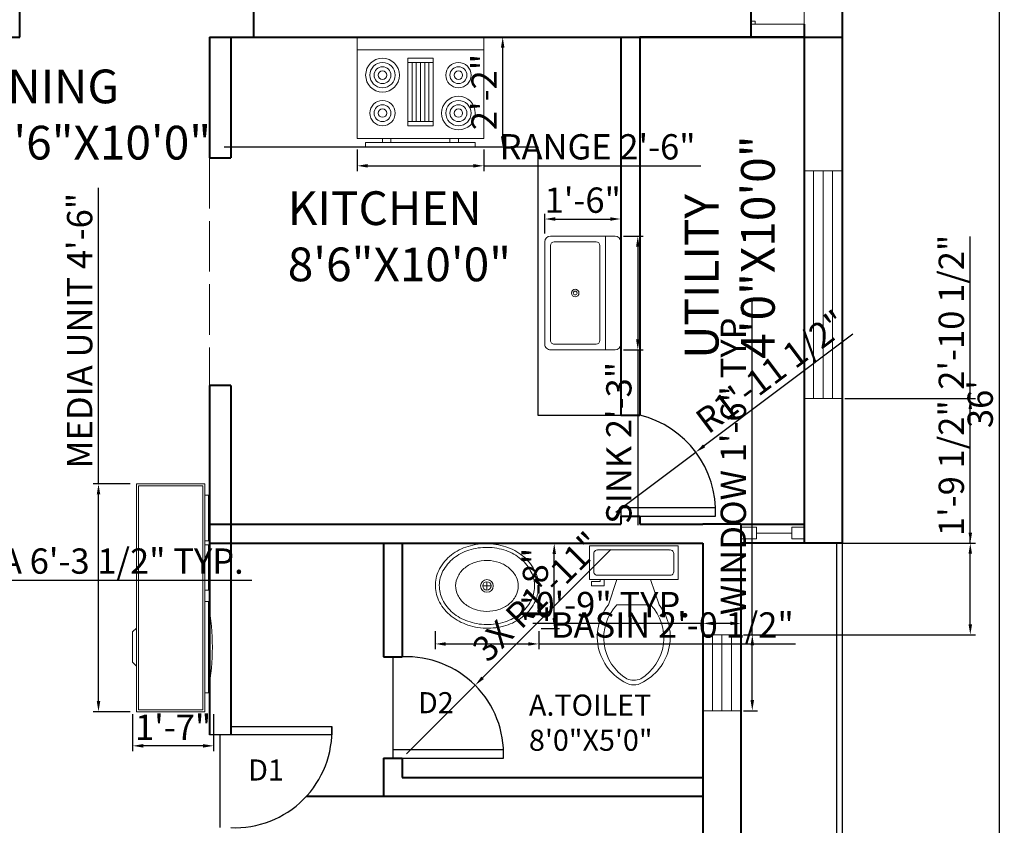
# Model space of a CAD drawing. Units: inches. Extents: x 459864 to 460310, y 324185 to 324787.
# Tile 111 of 112: x 460076 to 460310, y 324400 to 324591. Entities that reach past the tile are written whole.
import ezdxf

# ---------------------------------------------------------------- set-up
doc = ezdxf.new("R2010")
doc.units = ezdxf.units.IN
doc.linetypes.add('ACAD_ISO02W100', pattern=[15, 12, -3])
for name, color, linetype, lineweight in [('A-ANNO-DIMS', 2, 'Continuous', 18), ('A-ANNO-TEXT', 7, 'Continuous', 18), ('A-AREA-IDEN', 7, 'Continuous', 25), ('A-DOOR', 3, 'Continuous', 25), ('A-EQPM', 9, 'Continuous', 18), ('A-FLOR-CASE', 8, 'Continuous', 25), ('A-FLOR-FIXT', 9, 'Continuous', 18), ('A-FURN', 8, 'Continuous', 18), ('A-GLAZ', 4, 'Continuous', 18), ('A-WALL', 7, 'Continuous', 40), ('A-WALL-OVHD', 7, 'ACAD_ISO02W100', 18), ('C-PROP', 7, 'Continuous', 30)]:
    doc.layers.add(name, color=color, linetype=linetype, lineweight=lineweight)
doc.styles.get("Standard").update_dxf_attribs({"font": 'arial.ttf'})
doc.dimstyles.new('ISO-25', dxfattribs={"dimtxt": 6, "dimasz": 2.5, "dimexe": 1.25, "dimexo": 0.625, "dimtad": 1, "dimdec": 1, "dimlunit": 3, "dimtxsty": 'Standard', "dimcen": 2.5, "dimadec": 0, "dimazin": 0, "dimtfac": 1, "dimtdec": 1, "dimtmove": 0, "dimatfit": 3, "dimfxl": 1, "dimarcsym": 0})

# ---------------------------------------------------------------- blocks, each defined once
blk = doc.blocks.new('Window - Wood Frame 36 in. Wide plan')
for p, q in [((0, 6), (0, 0)), ((36, 6), (36, 0)), ((0, 4.5), (36, 4.5)), ((0, 3), (36, 3)), ((0, 1.5), (36, 1.5))]:
    blk.add_line(p, q)
blk = doc.blocks.new('Toilet - top')
for p, q in [((9.5, -6), (9.5, -2)), ((-10, -8.5), (-8, -8.5)), ((-10, -9.5), (-10, -8.5)), ((-8, -8.5), (-8, -8)), ((-7, -8), (-7, -9.5)), ((-4, -8), (-6, -14)), ((4, -8), (6, -14)), ((-7, -9.5), (-10, -9.5)), ((4, -14), (-4, -14))]:
    blk.add_line(p, q)
blk.add_lwpolyline([(10.5, -8), (10.5, 0), (-10.5, 0), (-10.5, -8)], close=True)
for points in [[(-9.5, -2), (-9.5, -6)], [(8.5, -1), (-8.5, -1)], [(-8.5, -7), (8.5, -7)]]:
    blk.add_lwpolyline(points)
for centre, radius, start, end in [((-8.62, -1.88), 0.884, 81.8699, 188.1301), ((8.62, -1.88), 0.884, 351.8699, 98.1301), ((-8.62, -6.12), 0.884, 171.8699, 278.1301), ((8.62, -6.12), 0.884, 261.8699, 8.1301), ((3.52, -21.58), 12.17, 141.4691, 247.9714), ((4.2, -21.82), 11.33, 136.3677, 238.9468), ((-3.52, -21.58), 12.17, 292.0284, 38.5307), ((-4.2, -21.82), 11.33, 301.053, 43.6321), ((0, -27.88), 4, 245.7318, 294.2682), ((0, -29), 4, 254.8605, 285.1395)]:
    blk.add_arc(centre, radius, start, end)
blk = doc.blocks.new('Sink - Oval top')
for p, q in [((-1, 0), (1, 0)), ((0, 1), (0, -1))]:
    blk.add_line(p, q)
for points in [[(-12.23, 0.39, 0.117634), (-11.46, -3.36, 0.104469), (-8.88, -6.8, 0.090016), (-5.08, -9.07, 0.08192), (-0.32, -10.02, 0.08192), (4.49, -9.38, 0.090016), (8.42, -7.36, 0.104469), (11.22, -4.09, 0.117634), (12.23, -0.39, 0.117634), (11.46, 3.36, 0.104469), (8.88, 6.8, 0.090016), (5.08, 9.07, 0.08192), (0.32, 10.02, 0.08192), (-4.49, 9.38, 0.090016), (-8.42, 7.36, 0.104469), (-11.22, 4.09, 0.117634)], [(-11.29, 0.16, 0.118622), (-10.52, -3.25, 0.104678), (-8.07, -6.36, 0.089562), (-4.54, -8.37, 0.081185), (-0.13, -9.15, 0.081185), (4.3, -8.49, 0.089562), (7.89, -6.58, 0.104678), (10.42, -3.55, 0.118622), (11.29, -0.16, 0.118622), (10.52, 3.25, 0.104678), (8.07, 6.36, 0.089562), (4.54, 8.37, 0.081185), (0.13, 9.15, 0.081185), (-4.3, 8.49, 0.089562), (-7.89, 6.58, 0.104678), (-10.42, 3.55, 0.118622)], [(-7.42, 0.08, 0.118283), (-6.91, -2.17, 0.104607), (-5.29, -4.21, 0.089718), (-2.97, -5.53, 0.081436), (-0.07, -6.04, 0.081436), (2.84, -5.59, 0.089718), (5.2, -4.33, 0.104607), (6.86, -2.32, 0.118283), (7.42, -0.08, 0.118283), (6.91, 2.17, 0.104607), (5.29, 4.21, 0.089718), (2.97, 5.53, 0.081436), (0.07, 6.04, 0.081436), (-2.84, 5.59, 0.089718), (-5.2, 4.33, 0.104607), (-6.86, 2.32, 0.118283)]]:
    blk.add_lwpolyline(points, format="xyb", close=True)
for radius in [1.5, 1]:
    blk.add_circle((0, 0), radius)
blk = doc.blocks.new('Range-Oven - 30 in top')
for p, q in [((0, -3), (30, -3)), ((12, -6), (18, -6)), ((13, -20), (13, -6)), ((14, -6), (14, -20)), ((15, -20), (15, -6)), ((16, -6), (16, -20)), ((17, -20), (17, -6)), ((18, -20), (12, -20)), ((6, -24), (6, -25)), ((8, -25), (8, -24)), ((22, -25), (22, -24)), ((24, -24), (24, -25))]:
    blk.add_line(p, q)
for points in [[(0, -24), (0, 0), (30, 0), (30, -24)], [(12, -21), (12, -5), (18, -5), (18, -21)], [(2, -26), (2, -25), (28, -25), (28, -26)]]:
    blk.add_lwpolyline(points, close=True)
for centre, radius in [((6, -9), 4), ((6, -9), 3), ((6, -9), 2), ((24, -9), 3), ((24, -9), 2), ((6, -9), 1), ((24, -9), 1), ((24, -18), 4), ((6, -18), 3), ((6, -18), 2), ((24, -18), 3), ((24, -18), 2), ((6, -18), 1), ((24, -18), 1)]:
    blk.add_circle(centre, radius)
blk = doc.blocks.new('Sink-single - 30 in top')
blk.add_line((-15, -3.999996), (15, -3.999996))
for points in [[(-13.5, 0), (13.5, 0)], [(-15, -18.499996), (-15, -1.5)], [(15, -1.5), (15, -18.499996)], [(-13.5, -17.499996), (-13.5, -6.499996)], [(-12.5, -5.499996), (12.5, -5.499996)], [(13.5, -6.499996), (13.5, -17.499996)], [(13.5, -19.999996), (-13.5, -19.999996)], [(12.5, -18.499996), (-12.5, -18.499996)]]:
    blk.add_lwpolyline(points)
for radius in [1, 0.5]:
    blk.add_circle((0, -11.999996), radius)
for centre, radius, start, end in [((-13.5, -1.5), 1.5, 90, 180), ((13.5, -1.5), 1.5, 0, 90), ((-12.5, -6.499996), 1, 90, 180), ((12.5, -6.499996), 1, 0, 90), ((-12.5, -17.499996), 1, 180, 270), ((12.5, -17.499996), 1, 270, 0), ((-13.5, -18.499996), 1.5, 180, 270), ((13.5, -18.499996), 1.5, 270, 0)]:
    blk.add_arc(centre, radius, start, end)
blk = doc.blocks.new('Entertainment Center')
for p, q in [((-4, 0), (-5, -1)), ((4, 0), (-4, 0)), ((5, -1), (4, 0)), ((-17, -19), (-17, -1)), ((-17, -1), (43, -1)), ((-16.5, -18.5), (-16.5, -1.5)), ((-16.5, -1.5), (42.5, -1.5)), ((42.5, -1.5), (42.5, -18.5)), ((43, -1), (43, -19)), ((43, -19), (-17, -19)), ((42.5, -18.5), (-16.5, -18.5)), ((-12, -20), (-12, -19)), ((12, -20), (-12, -20)), ((12, -19), (12, -20)), ((15, -20), (15, -19)), ((27, -20), (15, -20)), ((27, -19), (27, -20)), ((28, -20), (28, -19)), ((40, -20), (28, -20)), ((40, -19), (40, -20))]:
    blk.add_line(p, q)
blk.add_arc((0, 40), 61, 259.6111, 280.3889)
blk = doc.blocks.new('*D21')
at = {"layer": 'A-ANNO-DIMS', "color": 0, "lineweight": -2, "transparency": 16777216}
for p, q in [((460247.74, 324715.48), (460309.58, 324715.48)), ((460308.33, 324712.98), (460308.33, 324285.98)), ((460247.74, 324283.48), (460309.58, 324283.48))]:
    blk.add_line(p, q, dxfattribs=at)
at = {"layer": 'A-ANNO-DIMS', "color": 0, "transparency": 16777216}
for points in [[(460307.91, 324712.98), (460308.75, 324712.98), (460308.33, 324715.48)], [(460307.91, 324285.98), (460308.75, 324285.98), (460308.33, 324283.48)]]:
    blk.add_solid(points, dxfattribs=at)
at = {"layer": 'Defpoints', "color": 0, "transparency": 16777216}
for p in [(460247.11, 324715.48), (460247.11, 324283.48), (460308.33, 324283.48)]:
    blk.add_point(p, dxfattribs=at)
at = {"layer": 'A-ANNO-DIMS', "color": 0, "transparency": 16777216, "insert": (460304.64, 324499.48), "char_height": 6, "attachment_point": 5, "rotation": 90}
blk.add_mtext("36'", dxfattribs=at)
blk = doc.blocks.new('*D26')
at = {"layer": 'A-ANNO-DIMS', "color": 0, "lineweight": -2, "transparency": 16777216}
for p, q in [((460249.81, 324444.78), (460249.81, 324524.45)), ((460247.74, 324444.78), (460251.06, 324444.78)), ((460249.81, 324429.28), (460249.81, 324442.28)), ((460247.74, 324426.78), (460251.06, 324426.78))]:
    blk.add_line(p, q, dxfattribs=at)
at = {"layer": 'A-ANNO-DIMS', "color": 0, "transparency": 16777216}
for points in [[(460249.4, 324442.28), (460250.23, 324442.28), (460249.81, 324444.78)], [(460249.4, 324429.28), (460250.23, 324429.28), (460249.81, 324426.78)]]:
    blk.add_solid(points, dxfattribs=at)
at = {"layer": 'Defpoints', "color": 0, "transparency": 16777216}
for p in [(460247.11, 324444.78), (460249.81, 324444.78), (460247.11, 324426.78)]:
    blk.add_point(p, dxfattribs=at)
at = {"layer": 'A-ANNO-DIMS', "color": 0, "transparency": 16777216, "insert": (460246.09, 324485.87), "char_height": 6, "attachment_point": 5, "rotation": 90}
blk.add_mtext('WINDOW 1\'-6" TYP.', dxfattribs=at)
blk = doc.blocks.new('*D27')
at = {"layer": 'A-ANNO-DIMS', "color": 0, "lineweight": -2, "transparency": 16777216}
for p, q in [((460238.11, 324445.4), (460238.11, 324448.73)), ((460247.11, 324445.4), (460247.11, 324448.73)), ((460238.11, 324447.48), (460197.79, 324447.48)), ((460244.61, 324447.48), (460240.61, 324447.48))]:
    blk.add_line(p, q, dxfattribs=at)
at = {"layer": 'A-ANNO-DIMS', "color": 0, "transparency": 16777216}
for points in [[(460240.61, 324447.9), (460240.61, 324447.06), (460238.11, 324447.48)], [(460244.61, 324447.9), (460244.61, 324447.06), (460247.11, 324447.48)]]:
    blk.add_solid(points, dxfattribs=at)
at = {"layer": 'Defpoints', "color": 0, "transparency": 16777216}
for p in [(460238.11, 324447.48), (460238.11, 324444.78), (460247.11, 324444.78)]:
    blk.add_point(p, dxfattribs=at)
at = {"layer": 'A-ANNO-DIMS', "color": 0, "transparency": 16777216, "insert": (460216.7, 324451.17), "char_height": 6, "attachment_point": 5}
blk.add_mtext('0\'-9" TYP.', dxfattribs=at)
blk = doc.blocks.new('*D32')
at = {"layer": 'A-ANNO-DIMS', "color": 0, "lineweight": -2, "transparency": 16777216}
for p, q in [((459976.12, 324468.46), (459976.12, 324456.5)), ((460051.72, 324468.46), (460051.72, 324456.5)), ((459978.62, 324457.75), (460049.22, 324457.75)), ((460051.72, 324457.75), (460131.14, 324457.75))]:
    blk.add_line(p, q, dxfattribs=at)
at = {"layer": 'A-ANNO-DIMS', "color": 0, "transparency": 16777216}
for points in [[(459978.62, 324458.17), (459978.62, 324457.33), (459976.12, 324457.75)], [(460049.22, 324458.17), (460049.22, 324457.33), (460051.72, 324457.75)]]:
    blk.add_solid(points, dxfattribs=at)
at = {"layer": 'Defpoints', "color": 0, "transparency": 16777216}
for p in [(459976.12, 324469.09), (460051.72, 324469.09), (460051.72, 324457.75)]:
    blk.add_point(p, dxfattribs=at)
at = {"layer": 'A-ANNO-DIMS', "color": 0, "transparency": 16777216, "insert": (460092.68, 324461.48), "char_height": 6, "attachment_point": 5}
blk.add_mtext('SOFA 6\'-3 1/2" TYP.', dxfattribs=at)
blk = doc.blocks.new('*D42')
at = {"layer": 'A-ANNO-DIMS', "color": 0, "lineweight": -2, "transparency": 16777216}
for p, q in [((460174.61, 324445.66), (460174.61, 324441.36)), ((460199.16, 324445.66), (460199.16, 324441.36)), ((460177.11, 324442.61), (460196.66, 324442.61)), ((460199.16, 324442.61), (460260.06, 324442.61))]:
    blk.add_line(p, q, dxfattribs=at)
at = {"layer": 'A-ANNO-DIMS', "color": 0, "transparency": 16777216}
for points in [[(460177.11, 324443.02), (460177.11, 324442.19), (460174.61, 324442.61)], [(460196.66, 324443.02), (460196.66, 324442.19), (460199.16, 324442.61)]]:
    blk.add_solid(points, dxfattribs=at)
at = {"layer": 'Defpoints', "color": 0, "transparency": 16777216}
for p in [(460174.61, 324446.29), (460199.16, 324446.29), (460199.16, 324442.61)]:
    blk.add_point(p, dxfattribs=at)
at = {"layer": 'A-ANNO-DIMS', "color": 0, "transparency": 16777216, "insert": (460230.86, 324446.33), "char_height": 6, "attachment_point": 5}
blk.add_mtext('BASIN 2\'-0 1/2"', dxfattribs=at)
blk = doc.blocks.new('*D43')
at = {"layer": 'A-ANNO-DIMS', "color": 0, "lineweight": -2, "transparency": 16777216}
for p, q in [((460199.78, 324466.43), (460204.09, 324466.43)), ((460202.84, 324448.79), (460202.84, 324463.93)), ((460199.78, 324446.29), (460204.09, 324446.29))]:
    blk.add_line(p, q, dxfattribs=at)
at = {"layer": 'A-ANNO-DIMS', "color": 0, "transparency": 16777216}
for points in [[(460202.43, 324463.93), (460203.26, 324463.93), (460202.84, 324466.43)], [(460202.43, 324448.79), (460203.26, 324448.79), (460202.84, 324446.29)]]:
    blk.add_solid(points, dxfattribs=at)
at = {"layer": 'Defpoints', "color": 0, "transparency": 16777216}
for p in [(460199.16, 324466.43), (460202.84, 324466.43), (460199.16, 324446.29)]:
    blk.add_point(p, dxfattribs=at)
at = {"layer": 'A-ANNO-DIMS', "color": 0, "transparency": 16777216, "insert": (460199.15, 324456.36), "char_height": 6, "attachment_point": 5, "rotation": 90}
blk.add_mtext('1\'-8"', dxfattribs=at)
blk = doc.blocks.new('*D48')
at = {"layer": 'A-ANNO-DIMS', "color": 0, "lineweight": -2, "transparency": 16777216}
for p, q in [((460156.12, 324559.86), (460156.12, 324554.73)), ((460186.12, 324559.86), (460186.12, 324554.73)), ((460158.62, 324555.98), (460183.62, 324555.98)), ((460186.12, 324555.98), (460237.64, 324555.98))]:
    blk.add_line(p, q, dxfattribs=at)
at = {"layer": 'A-ANNO-DIMS', "color": 0, "transparency": 16777216}
for points in [[(460158.62, 324556.4), (460158.62, 324555.57), (460156.12, 324555.98)], [(460183.62, 324556.4), (460183.62, 324555.57), (460186.12, 324555.98)]]:
    blk.add_solid(points, dxfattribs=at)
at = {"layer": 'Defpoints', "color": 0, "transparency": 16777216}
for p in [(460156.12, 324560.48), (460186.12, 324560.48), (460186.12, 324555.98)]:
    blk.add_point(p, dxfattribs=at)
at = {"layer": 'A-ANNO-DIMS', "color": 0, "transparency": 16777216, "insert": (460213.13, 324559.71), "char_height": 6, "attachment_point": 5}
blk.add_mtext('RANGE 2\'-6"', dxfattribs=at)
blk = doc.blocks.new('*D49')
at = {"layer": 'A-ANNO-DIMS', "color": 0, "lineweight": -2, "transparency": 16777216}
for p, q in [((460186.74, 324586.48), (460191.87, 324586.48)), ((460190.62, 324562.98), (460190.62, 324583.98)), ((460186.74, 324560.48), (460191.87, 324560.48))]:
    blk.add_line(p, q, dxfattribs=at)
at = {"layer": 'A-ANNO-DIMS', "color": 0, "transparency": 16777216}
for points in [[(460190.2, 324583.98), (460191.03, 324583.98), (460190.62, 324586.48)], [(460190.2, 324562.98), (460191.03, 324562.98), (460190.62, 324560.48)]]:
    blk.add_solid(points, dxfattribs=at)
at = {"layer": 'Defpoints', "color": 0, "transparency": 16777216}
for p in [(460186.12, 324586.48), (460190.62, 324586.48), (460186.12, 324560.48)]:
    blk.add_point(p, dxfattribs=at)
at = {"layer": 'A-ANNO-DIMS', "color": 0, "transparency": 16777216, "insert": (460186.98, 324573.48), "char_height": 6, "attachment_point": 5, "rotation": 90}
blk.add_mtext('2\'-2"', dxfattribs=at)
blk = doc.blocks.new('*D50')
at = {"layer": 'A-ANNO-DIMS', "color": 0, "lineweight": -2, "transparency": 16777216}
for p, q in [((460219.24, 324539.32), (460223.91, 324539.32)), ((460222.66, 324536.82), (460222.66, 324514.82)), ((460219.24, 324512.32), (460223.91, 324512.32)), ((460222.66, 324512.32), (460222.66, 324470.76))]:
    blk.add_line(p, q, dxfattribs=at)
at = {"layer": 'A-ANNO-DIMS', "color": 0, "transparency": 16777216}
for points in [[(460222.25, 324536.82), (460223.08, 324536.82), (460222.66, 324539.32)], [(460222.25, 324514.82), (460223.08, 324514.82), (460222.66, 324512.32)]]:
    blk.add_solid(points, dxfattribs=at)
at = {"layer": 'Defpoints', "color": 0, "transparency": 16777216}
for p in [(460218.61, 324539.32), (460218.61, 324512.32), (460222.66, 324512.32)]:
    blk.add_point(p, dxfattribs=at)
at = {"layer": 'A-ANNO-DIMS', "color": 0, "transparency": 16777216, "insert": (460218.94, 324490.29), "char_height": 6, "attachment_point": 5, "rotation": 90}
blk.add_mtext('SINK 2\'-3"', dxfattribs=at)
blk = doc.blocks.new('*D51')
at = {"layer": 'A-ANNO-DIMS', "color": 0, "lineweight": -2, "transparency": 16777216}
for p, q in [((460200.61, 324539.95), (460200.61, 324544.62)), ((460218.61, 324539.95), (460218.61, 324544.62)), ((460203.11, 324543.37), (460216.11, 324543.37))]:
    blk.add_line(p, q, dxfattribs=at)
at = {"layer": 'A-ANNO-DIMS', "color": 0, "transparency": 16777216}
for points in [[(460203.11, 324543.79), (460203.11, 324542.95), (460200.61, 324543.37)], [(460216.11, 324543.79), (460216.11, 324542.95), (460218.61, 324543.37)]]:
    blk.add_solid(points, dxfattribs=at)
at = {"layer": 'Defpoints', "color": 0, "transparency": 16777216}
for p in [(460218.61, 324543.37), (460200.61, 324539.32), (460218.61, 324539.32)]:
    blk.add_point(p, dxfattribs=at)
at = {"layer": 'A-ANNO-DIMS', "color": 0, "transparency": 16777216, "insert": (460209.61, 324547.06), "char_height": 6, "attachment_point": 5}
blk.add_mtext('1\'-6"', dxfattribs=at)
blk = doc.blocks.new('*D52')
at = {"layer": 'A-ANNO-DIMS', "color": 0, "lineweight": -2, "transparency": 16777216}
for p, q in [((460094.76, 324480.55), (460094.76, 324550.73)), ((460102.24, 324480.55), (460093.51, 324480.55)), ((460094.76, 324429.05), (460094.76, 324478.05)), ((460102.24, 324426.55), (460093.51, 324426.55))]:
    blk.add_line(p, q, dxfattribs=at)
at = {"layer": 'A-ANNO-DIMS', "color": 0, "transparency": 16777216}
for points in [[(460094.35, 324478.05), (460095.18, 324478.05), (460094.76, 324480.55)], [(460094.35, 324429.05), (460095.18, 324429.05), (460094.76, 324426.55)]]:
    blk.add_solid(points, dxfattribs=at)
at = {"layer": 'Defpoints', "color": 0, "transparency": 16777216}
for p in [(460094.76, 324480.55), (460102.86, 324480.55), (460102.86, 324426.55)]:
    blk.add_point(p, dxfattribs=at)
at = {"layer": 'A-ANNO-DIMS', "color": 0, "transparency": 16777216, "insert": (460091.07, 324516.89), "char_height": 6, "attachment_point": 5, "rotation": 90}
blk.add_mtext('MEDIA UNIT 4\'-6"', dxfattribs=at)
blk = doc.blocks.new('*D53')
at = {"layer": 'A-ANNO-DIMS', "color": 0, "lineweight": -2, "transparency": 16777216}
for p, q in [((460102.86, 324425.92), (460102.86, 324417.2)), ((460122.06, 324425.92), (460122.06, 324417.2)), ((460119.56, 324418.45), (460105.36, 324418.45))]:
    blk.add_line(p, q, dxfattribs=at)
at = {"layer": 'A-ANNO-DIMS', "color": 0, "transparency": 16777216}
for points in [[(460105.36, 324418.86), (460105.36, 324418.03), (460102.86, 324418.45)], [(460119.56, 324418.86), (460119.56, 324418.03), (460122.06, 324418.45)]]:
    blk.add_solid(points, dxfattribs=at)
at = {"layer": 'Defpoints', "color": 0, "transparency": 16777216}
for p in [(460102.86, 324426.55), (460122.06, 324426.55), (460102.86, 324418.45)]:
    blk.add_point(p, dxfattribs=at)
at = {"layer": 'A-ANNO-DIMS', "color": 0, "transparency": 16777216, "insert": (460112.46, 324422.09), "char_height": 6, "attachment_point": 5}
blk.add_mtext('1\'-7"', dxfattribs=at)
blk = doc.blocks.new('*D63')
at = {"layer": 'A-ANNO-DIMS', "color": 0, "lineweight": -2, "transparency": 16777216}
for p, q in [((460301.51, 324466.48), (460301.51, 324499.6)), ((460247.74, 324466.48), (460302.76, 324466.48)), ((460301.51, 324447.28), (460301.51, 324463.98)), ((460247.74, 324444.78), (460302.76, 324444.78))]:
    blk.add_line(p, q, dxfattribs=at)
at = {"layer": 'A-ANNO-DIMS', "color": 0, "transparency": 16777216}
for points in [[(460301.1, 324463.98), (460301.93, 324463.98), (460301.51, 324466.48)], [(460301.1, 324447.28), (460301.93, 324447.28), (460301.51, 324444.78)]]:
    blk.add_solid(points, dxfattribs=at)
at = {"layer": 'Defpoints', "color": 0, "transparency": 16777216}
for p in [(460247.11, 324466.48), (460301.51, 324466.48), (460247.11, 324444.78)]:
    blk.add_point(p, dxfattribs=at)
at = {"layer": 'A-ANNO-DIMS', "color": 0, "transparency": 16777216, "insert": (460297.79, 324484.29), "char_height": 6, "attachment_point": 5, "rotation": 90}
blk.add_mtext('1\'-9 1/2"', dxfattribs=at)
blk = doc.blocks.new('*D64')
at = {"layer": 'A-ANNO-DIMS', "color": 0, "lineweight": -2, "transparency": 16777216}
for p, q in [((460301.51, 324500.8), (460301.51, 324539.24)), ((460271.74, 324500.8), (460302.76, 324500.8)), ((460301.51, 324468.98), (460301.51, 324498.3)), ((460271.74, 324466.48), (460302.76, 324466.48))]:
    blk.add_line(p, q, dxfattribs=at)
at = {"layer": 'A-ANNO-DIMS', "color": 0, "transparency": 16777216}
for points in [[(460301.1, 324498.3), (460301.93, 324498.3), (460301.51, 324500.8)], [(460301.1, 324468.98), (460301.93, 324468.98), (460301.51, 324466.48)]]:
    blk.add_solid(points, dxfattribs=at)
at = {"layer": 'Defpoints', "color": 0, "transparency": 16777216}
for p in [(460271.11, 324500.8), (460301.51, 324500.8), (460271.11, 324466.48)]:
    blk.add_point(p, dxfattribs=at)
at = {"layer": 'A-ANNO-DIMS', "color": 0, "transparency": 16777216, "insert": (460297.79, 324521.27), "char_height": 6, "attachment_point": 5, "rotation": 90}
blk.add_mtext('2\'-10 1/2"', dxfattribs=at)
blk = doc.blocks.new('*D72')
at = {"layer": 'A-ANNO-DIMS', "color": 0, "lineweight": -2, "transparency": 16777216}
for p, q in [((460216.26, 324464.99), (460185.86, 324434.59)), ((460167.81, 324416.54), (460184.09, 324432.82))]:
    blk.add_line(p, q, dxfattribs=at)
at = {"layer": 'A-ANNO-DIMS', "color": 0, "transparency": 16777216}
blk.add_solid([(460185.57, 324434.88), (460186.16, 324434.29), (460184.09, 324432.82)], dxfattribs=at)
at = {"layer": 'Defpoints', "color": 0, "transparency": 16777216}
for p in [(460184.09, 324432.82), (460167.81, 324416.54)]:
    blk.add_point(p, dxfattribs=at)
at = {"layer": 'A-ANNO-DIMS', "color": 0, "transparency": 16777216, "insert": (460199.33, 324453.28), "char_height": 6, "attachment_point": 5, "rotation": 45.0013}
blk.add_mtext('3X R1\'-11"', dxfattribs=at)
blk = doc.blocks.new('*D74')
at = {"layer": 'A-ANNO-DIMS', "color": 0, "lineweight": -2, "transparency": 16777216}
for p, q in [((460273.67, 324516.03), (460238.4, 324489.58)), ((460217.45, 324473.87), (460236.4, 324488.08))]:
    blk.add_line(p, q, dxfattribs=at)
at = {"layer": 'A-ANNO-DIMS', "color": 0, "transparency": 16777216}
blk.add_solid([(460238.15, 324489.91), (460238.65, 324489.24), (460236.4, 324488.08)], dxfattribs=at)
at = {"layer": 'Defpoints', "color": 0, "transparency": 16777216}
for p in [(460236.4, 324488.08), (460217.45, 324473.87)]:
    blk.add_point(p, dxfattribs=at)
at = {"layer": 'A-ANNO-DIMS', "color": 0, "transparency": 16777216, "insert": (460254.8, 324506.54), "char_height": 6, "attachment_point": 5, "rotation": 36.8704}
blk.add_mtext('R1\'-11 1/2"', dxfattribs=at)

msp = doc.modelspace()

# ---------------------------------------------------------------- linework, layer by layer
at = {"layer": 'A-DOOR'}
for p, q in [((460241.11, 324474.87), (460218.61, 324474.87)), ((460218.61, 324474.87), (460218.61, 324472.87)), ((460241.11, 324472.87), (460241.11, 324474.87)), ((460223.11, 324472.87), (460241.11, 324472.87)), ((460164.56, 324439.54), (460164.56, 324415.54)), ((460126.11, 324423.05), (460150.11, 324423.05)), ((460150.11, 324423.05), (460150.11, 324421.05)), ((460150.11, 324421.05), (460121.11, 324421.05)), ((460123.61, 324399.05), (460123.61, 324421.05)), ((460190.81, 324417.54), (460164.56, 324417.54)), ((460166.81, 324415.54), (460190.81, 324415.54)), ((460190.81, 324415.54), (460190.81, 324417.54))]:
    msp.add_line(p, q, dxfattribs=at)
for centre, radius, start, end in [((460217.45, 324473.87), 23.69, 357.5805, 76.1593), ((460167.81, 324416.54), 23.02, 357.5104, 92.4896), ((460127.11, 324422.05), 23.02, 267.5104, 2.4896)]:
    msp.add_arc(centre, radius, start, end, dxfattribs=at)
at = {"layer": 'A-FLOR-CASE'}
for p, q in [((460124.6, 324560.48), (460198.97, 324560.48)), ((460198.97, 324560.48), (460198.97, 324496.87)), ((460198.97, 324496.87), (460218.61, 324496.87))]:
    msp.add_line(p, q, dxfattribs=at)
at = {"layer": 'A-GLAZ'}
for p, q in [((460249.48, 324589.6), (460249.48, 324590.28)), ((460249.48, 324590.28), (460250.49, 324590.28)), ((460262.11, 324589.6), (460249.48, 324589.6)), ((460250.49, 324590.28), (460250.49, 324589.6)), ((460250.82, 324470.28), (460247.11, 324470.28)), ((460250.82, 324470.28), (460250.82, 324467.53)), ((460262.11, 324470.28), (460259.18, 324470.28)), ((460259.18, 324470.28), (460259.18, 324467.53)), ((460250.82, 324467.53), (460247.11, 324467.53)), ((460250.82, 324468.91), (460259.18, 324468.91)), ((460259.18, 324467.53), (460262.11, 324467.53))]:
    msp.add_line(p, q, dxfattribs=at)
at = {"layer": 'A-WALL'}
for p, q in [((460076.11, 324586.48), (460076.11, 324646.48)), ((460131.61, 324586.48), (460131.61, 324598.49)), ((460249.48, 324595.48), (460249.48, 324586.48)), ((460271.11, 324595.48), (460271.11, 324466.48)), ((460262.11, 324589.6), (460262.11, 324466.48)), ((460064.71, 324586.48), (460076.11, 324586.48)), ((460121.11, 324586.48), (460238.11, 324586.48)), ((460121.11, 324586.48), (460121.11, 324557.89)), ((460126.11, 324586.48), (460126.11, 324557.89)), ((460218.61, 324586.48), (460218.61, 324496.87)), ((460262.11, 324586.48), (460223.11, 324586.48)), ((460223.11, 324586.48), (460223.11, 324496.87)), ((460238.11, 324586.48), (460247.11, 324586.48)), ((460247.11, 324586.48), (460271.11, 324586.48)), ((460121.11, 324557.89), (460126.11, 324557.89)), ((460126.11, 324503.88), (460121.11, 324503.88)), ((460121.11, 324503.88), (460121.11, 324466.48)), ((460126.11, 324503.88), (460126.11, 324466.48)), ((460218.61, 324496.87), (460223.11, 324496.87)), ((460218.61, 324472.87), (460223.11, 324472.87)), ((460218.61, 324472.87), (460218.61, 324470.98)), ((460223.11, 324472.87), (460223.11, 324470.98)), ((460121.11, 324470.98), (460218.61, 324470.98)), ((460223.11, 324470.98), (460238.11, 324470.98)), ((460247.11, 324470.98), (460238.11, 324470.98)), ((460247.11, 324470.98), (460247.11, 324283.48)), ((460247.11, 324470.98), (460262.11, 324470.98)), ((460121.11, 324466.48), (460238.11, 324466.48)), ((460121.11, 324466.48), (460121.11, 324421.05)), ((460126.11, 324466.48), (460126.11, 324421.05)), ((460162.31, 324466.48), (460162.31, 324439.54)), ((460166.81, 324466.48), (460166.81, 324439.54)), ((460223.11, 324466.48), (460238.11, 324466.48)), ((460238.11, 324466.48), (460238.11, 324292.48)), ((460262.11, 324466.48), (460247.11, 324466.48)), ((460271.11, 324466.48), (460262.11, 324466.48)), ((460162.31, 324439.54), (460166.81, 324439.54)), ((460162.31, 324415.54), (460166.81, 324415.54)), ((460162.31, 324415.54), (460162.31, 324406.48)), ((460166.81, 324415.54), (460166.81, 324410.98)), ((460166.81, 324410.98), (460238.11, 324410.98)), ((460144.08, 324406.48), (460238.11, 324406.48))]:
    msp.add_line(p, q, dxfattribs=at)
at = {"layer": 'A-WALL-OVHD'}
for p, q in [((460262.11, 324586.48), (460262.11, 324595.48)), ((460121.11, 324557.89), (460121.11, 324503.88))]:
    msp.add_line(p, q, dxfattribs=at)
at = {"layer": 'C-PROP'}
for p, q in [((460269.8, 324466.48), (460269.8, 324199.48)), ((460271.11, 324466.48), (460271.11, 324194.95))]:
    msp.add_line(p, q, dxfattribs=at)

# ---------------------------------------------------------------- block references
at = {"layer": 'A-EQPM'}
msp.add_blockref('Range-Oven - 30 in top', (460156.12, 324586.48), dxfattribs=at)
at = {"layer": 'A-FLOR-FIXT', "xscale": 0.9, "yscale": 0.9, "rotation": 270}
msp.add_blockref('Sink-single - 30 in top', (460218.61, 324525.82), dxfattribs=at)
at = {"layer": 'A-FLOR-FIXT'}
for name, p in [('Sink - Oval top', (460186.88, 324456.36)), ('Toilet - top', (460221.7, 324465.89))]:
    msp.add_blockref(name, p, dxfattribs=at)
at = {"layer": 'A-FURN', "xscale": 0.9, "yscale": 0.9, "rotation": 90}
msp.add_blockref('Entertainment Center', (460102.86, 324441.85), dxfattribs=at)
at = {"layer": 'A-GLAZ', "yscale": 1.5, "zscale": 1.5, "rotation": 90}
for p, xscale in [((460271.11, 324500.8), 1.5), ((460247.11, 324426.78), 0.5)]:
    msp.add_blockref('Window - Wood Frame 36 in. Wide plan', p, dxfattribs=dict(at, xscale=xscale))

# ---------------------------------------------------------------- texts
at = {"layer": 'A-ANNO-TEXT', "char_height": 5, "attachment_point": 1}
for s, insert in [('D2', (460170.52, 324431.18)), ('D1', (460130.25, 324415.22))]:
    msp.add_mtext(s, dxfattribs=dict(at, insert=insert))
at = {"layer": 'A-AREA-IDEN', "char_height": 8, "width": 75.646, "attachment_point": 1}
for s, insert in [('DINING\\P14\'6"X10\'0"', (460062.45, 324578.81)), ('KITCHEN\\P8\'6"X10\'0"', (460139.64, 324549.94))]:
    msp.add_mtext(s, dxfattribs=dict(at, insert=insert))
at = {"layer": 'A-AREA-IDEN', "insert": (460233.81, 324510.22), "char_height": 8, "width": 75.646, "attachment_point": 1, "rotation": 90}
msp.add_mtext('UTILITY\\P4\'0"X10\'0"', dxfattribs=at)
at = {"layer": 'A-AREA-IDEN', "insert": (460196.84, 324430.61), "char_height": 5, "attachment_point": 1}
msp.add_mtext('A.TOILET\\P8\'0"X5\'0"', dxfattribs=at)

# ---------------------------------------------------------------- dimensions: what is measured, and where the dimension line sits
at = {"layer": 'A-ANNO-DIMS'}
for base, p1, p2, angle, override, picture, middle in [((460308.33, 324283.48), (460247.11, 324715.48), (460247.11, 324283.48), 90, {"dimclrd": 0, "dimclre": 0, "dimclrt": 0}, '*D21', (460304.64, 324499.48)), ((460190.62, 324586.48), (460186.12, 324560.48), (460186.12, 324586.48), 90, {"dimdec": 1, "dimlfac": 1, "dimrnd": 0, "dimzin": 1, "dimdsep": 46, "dimlunit": 4, "dimfrac": 2}, '*D49', (460186.98, 324573.48)), ((460301.51, 324500.8), (460271.11, 324466.48), (460271.11, 324500.8), 90, {"dimdec": 1, "dimlfac": 1, "dimrnd": 0, "dimzin": 1, "dimdsep": 46, "dimlunit": 4, "dimfrac": 2}, '*D64', (460297.79, 324521.27)), ((460301.51, 324466.48), (460247.11, 324444.78), (460247.11, 324466.48), 90, {"dimdec": 1, "dimlfac": 1, "dimrnd": 0, "dimzin": 1, "dimdsep": 46, "dimlunit": 4, "dimfrac": 2}, '*D63', (460297.79, 324484.29)), ((460202.84, 324466.43), (460199.16, 324446.29), (460199.16, 324466.43), 90, {"dimdec": 1, "dimlfac": 1, "dimrnd": 0, "dimzin": 1, "dimdsep": 46, "dimlunit": 4, "dimfrac": 2}, '*D43', (460199.15, 324456.36)), ((460102.86, 324418.45), (460122.06, 324426.55), (460102.86, 324426.55), 180, {"dimdec": 1, "dimlfac": 1, "dimrnd": 0, "dimzin": 1, "dimdsep": 46, "dimlunit": 4, "dimfrac": 2}, '*D53', (460112.46, 324422.09))]:
    dim = msp.add_linear_dim(base=base, p1=p1, p2=p2, angle=angle, dimstyle='ISO-25', override=override, dxfattribs=at)
    dim.commit()
    dim.dimension.update_dxf_attribs({"geometry": picture, "text_midpoint": middle})
for base, p1, p2, text, picture, middle in [((460186.12, 324555.98), (460156.12, 324560.48), (460186.12, 324560.48), 'RANGE <>', '*D48', (460213.13, 324559.71)), ((460051.72, 324457.75), (459976.12, 324469.09), (460051.72, 324469.09), 'SOFA <> TYP.', '*D32', (460092.68, 324461.48)), ((460199.1596, 324442.6062), (460174.6087, 324446.2888), (460199.1596, 324446.2888), 'BASIN <>', '*D42', (460230.8583, 324446.3335))]:
    dim = msp.add_linear_dim(base=base, p1=p1, p2=p2, text=text, dimstyle='ISO-25', override={"dimdec": 1, "dimlfac": 1, "dimrnd": 0, "dimzin": 1, "dimdsep": 46, "dimlunit": 4, "dimfrac": 2}, dxfattribs=at)
    dim.commit()
    dim.dimension.update_dxf_attribs({"geometry": picture, "text_midpoint": middle})
dim = msp.add_linear_dim(base=(460218.61, 324543.37), p1=(460200.61, 324539.32), p2=(460218.61, 324539.32), dimstyle='ISO-25', override={"dimdec": 1, "dimlfac": 1, "dimrnd": 0, "dimzin": 1, "dimdsep": 46, "dimlunit": 4, "dimfrac": 2}, dxfattribs=at)
dim.commit()
dim.dimension.update_dxf_attribs({"geometry": '*D51', "text_midpoint": (460209.61, 324547.06)})
for base, p1, p2, angle, text, picture, middle in [((460094.76, 324480.55), (460102.86, 324426.55), (460102.86, 324480.55), 90, 'MEDIA UNIT <>', '*D52', (460091.07, 324516.89)), ((460222.66, 324512.32), (460218.61, 324539.32), (460218.61, 324512.32), 270, 'SINK <>', '*D50', (460218.94, 324490.29)), ((460249.81, 324444.78), (460247.11, 324426.78), (460247.11, 324444.78), 90, 'WINDOW <> TYP.', '*D26', (460246.09, 324485.87)), ((460238.11, 324447.48), (460247.11, 324444.78), (460238.11, 324444.78), 180, '<> TYP.', '*D27', (460216.7, 324451.17))]:
    dim = msp.add_linear_dim(base=base, p1=p1, p2=p2, angle=angle, text=text, dimstyle='ISO-25', override={"dimdec": 1, "dimlfac": 1, "dimrnd": 0, "dimzin": 1, "dimdsep": 46, "dimlunit": 4, "dimfrac": 2}, dxfattribs=at)
    dim.commit()
    dim.dimension.update_dxf_attribs({"geometry": picture, "text_midpoint": middle})
dim = msp.add_radius_dim(center=(460217.45, 324473.87), mpoint=(460236.4, 324488.08), dimstyle='ISO-25', override={"dimdec": 1, "dimlfac": 1, "dimrnd": 0, "dimzin": 1, "dimdsep": 46, "dimlunit": 4, "dimfrac": 2}, dxfattribs=at)
dim.commit()
dim.dimension.update_dxf_attribs({"geometry": '*D74', "text_midpoint": (460254.8, 324506.54)})
dim = msp.add_radius_dim(center=(460167.81, 324416.54), mpoint=(460184.09, 324432.82), text='3X <>', dimstyle='ISO-25', override={"dimdec": 1, "dimlfac": 1, "dimrnd": 0, "dimzin": 1, "dimdsep": 46, "dimlunit": 4, "dimfrac": 2}, dxfattribs=at)
dim.commit()
dim.dimension.update_dxf_attribs({"geometry": '*D72', "text_midpoint": (460199.33, 324453.28)})

doc.saveas('drawing.dxf')
